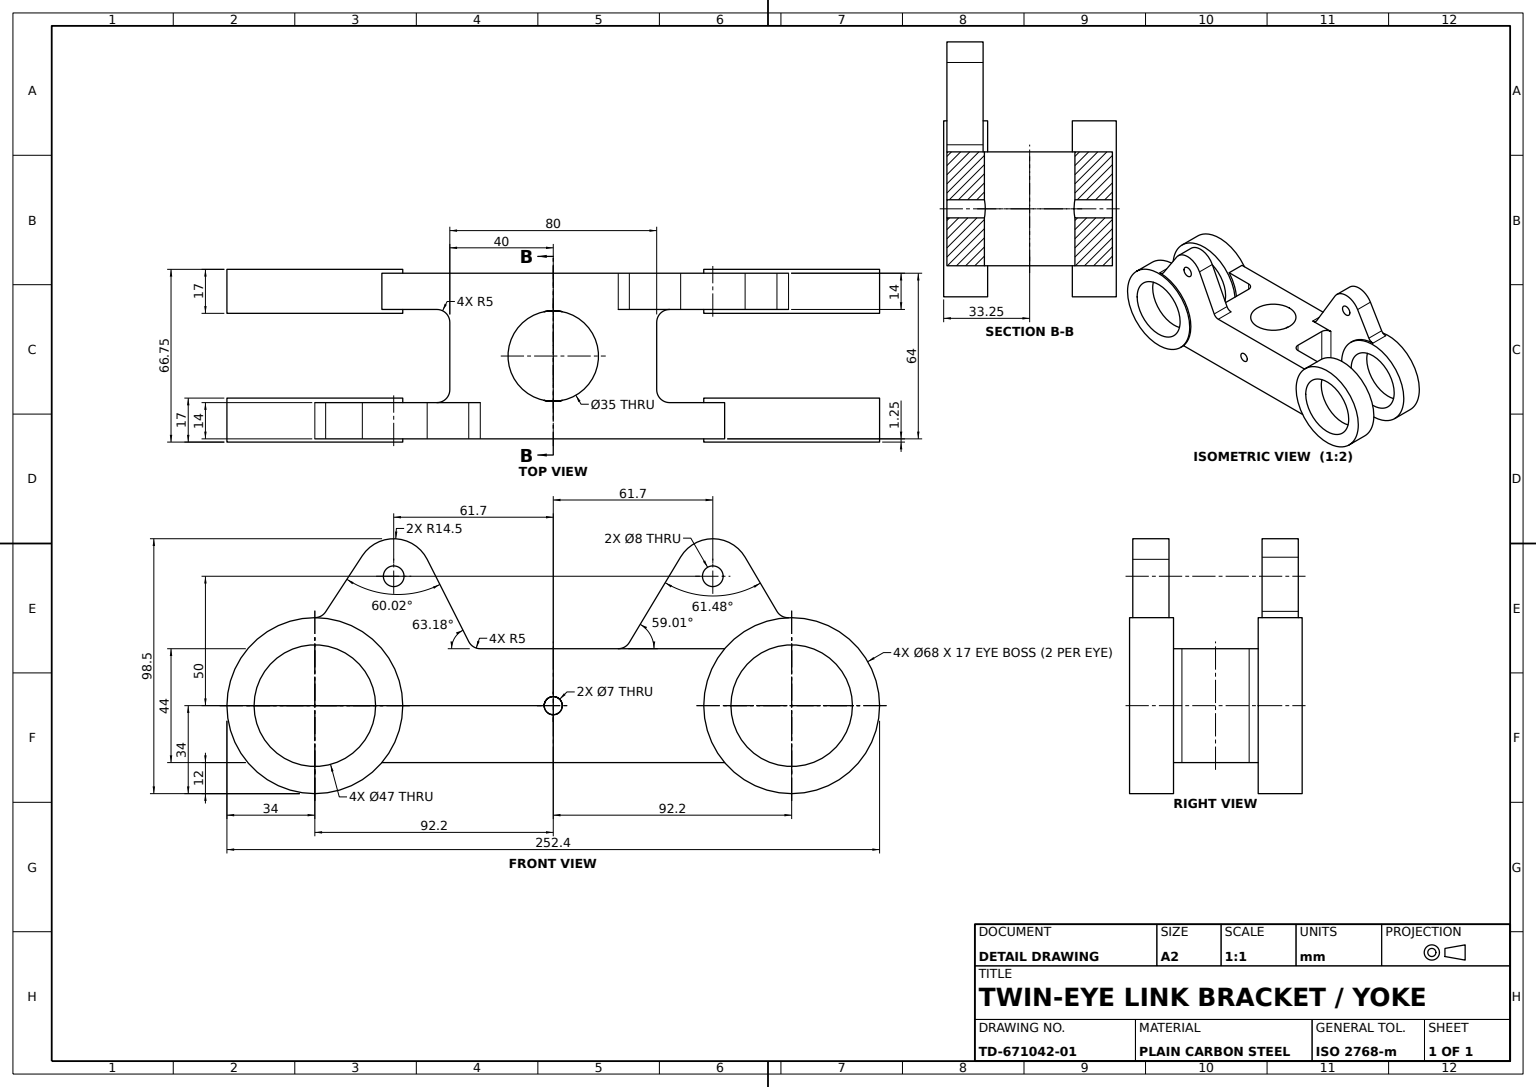
from build123d import *

# Parameters (mm, degrees)
CENTER_BODY_SKETCH_W         = 80
CENTER_BODY_SKETCH_H         = 64
CENTER_BODY_SKETCH_R         = 17.5
CENTER_BODY_DEPTH            = 44
PIVOT_EYES_SKETCH_R          = 34
PIVOT_EYES_SKETCH_R_2        = 23.5
PIVOT_EYES_68X_47_DEPTH      = 15.75
PIVOT_EYES_68X_47_2_DEPTH    = 15.75
EYE_FACE_PADS_SKETCH_R       = 34
EYE_FACE_PADS_SKETCH_R_2     = 23.5
EYE_FACE_PADS_DEPTH          = 1.25
MOUNTING_LUG_A_SKETCH_W      = 27.466221721
MOUNTING_LUG_A_SKETCH_H      = 44
MOUNTING_LUG_A_SKETCH_R      = 4
MOUNTING_LUG_A_DEPTH         = 7
MOUNTING_START               = -14
MOUNTING_LUG_B_SKETCH_R      = 4
MOUNTING_LUG_B_DEPTH         = 14
OFFSET_PIVOT_EYES_SKETCH_R   = 34
OFFSET_PIVOT_EYES_SKETCH_R_2 = 23.5
OFFSET_PIVOT_EYES_DEPTH      = 8.5
CENTER_WEB_SKETCH_W          = 28.251394121
CENTER_WEB_SKETCH_H          = 44
CENTER_WEB_DEPTH             = 14
PIN_HOLE_SKETCH_R            = 3.5
PIN_HOLE_7_DEPTH             = 200
LUG_A_FILLETS_R5_R           = 5
LUG_B_FILLETS_R5_R           = 5


with BuildPart() as part:
    # Center Body Sketch → Center Body (new body)
    with BuildSketch(Plane(origin=(0, 0, 0), x_dir=(1, 0, 0), z_dir=(0, 1, 0))):
        Rectangle(CENTER_BODY_SKETCH_W, CENTER_BODY_SKETCH_H)
        with Locations(Location((0, 0, 0), (0, 0, 270))):
            Circle(CENTER_BODY_SKETCH_R, mode=Mode.SUBTRACT)
    extrude(amount=CENTER_BODY_DEPTH)



with BuildPart() as body_2:
    # Pivot Eyes Sketch → Pivot Eyes Ø68xØ47 (new body)
    with BuildSketch(Plane.XY.offset(32)):
        with Locations((-92.2, 22)):
            Circle(PIVOT_EYES_SKETCH_R)
        with Locations((-92.2, 22)):
            Circle(PIVOT_EYES_SKETCH_R_2, mode=Mode.SUBTRACT)
    extrude(amount=-PIVOT_EYES_68X_47_DEPTH)



with BuildPart() as body_3:
    # Pivot Eyes Sketch → Pivot Eyes _68x_47 2 (new body)
    with BuildSketch(Plane.XY.offset(32)):
        with Locations((92.2, 22)):
            Circle(PIVOT_EYES_SKETCH_R)
        with Locations((92.2, 22)):
            Circle(PIVOT_EYES_SKETCH_R_2, mode=Mode.SUBTRACT)
    extrude(amount=-PIVOT_EYES_68X_47_2_DEPTH)


with BuildPart() as body_2_1:
    add(body_2.part)

    add(body_3.part)  # Eye Face Pads merges body 3
    # Eye Face Pads Sketch → Eye Face Pads (add)
    # profile 1 of 2: a face of its own
    with BuildSketch(Plane.XY.offset(32)):
        with Locations((-92.2, 22)):
            Circle(EYE_FACE_PADS_SKETCH_R)
        with Locations((-92.2, 22)):
            Circle(EYE_FACE_PADS_SKETCH_R_2, mode=Mode.SUBTRACT)
    # profile 2 of 2: a face of its own
    with BuildSketch(Plane.XY.offset(32)):
        with Locations((92.2, 22)):
            Circle(EYE_FACE_PADS_SKETCH_R)
        with Locations((92.2, 22)):
            Circle(EYE_FACE_PADS_SKETCH_R_2, mode=Mode.SUBTRACT)
    extrude(amount=EYE_FACE_PADS_DEPTH)


with BuildPart() as part_1:
    add(part.part)

    add(body_2_1.part)  # Mounting Lug A merges body 2
    # Mounting Lug A Sketch → Mounting Lug A (add, symmetric)
    # profile 1 of 2: a face of its own
    with BuildSketch(Plane.XY.offset(25)):
        with Locations((53.733110861, 22)):
            Rectangle(MOUNTING_LUG_A_SKETCH_W, MOUNTING_LUG_A_SKETCH_H)
    # profile 2 of 2: a face of its own
    with BuildSketch(Plane.XY.offset(25)):
        with BuildLine():
            Line((-40, 44), (-40, 0))
            Line((-40, 0), (-66.277037206, 0))
            ThreePointArc((-66.277037206, 0), (-61.345502759, 36.282856857), (-92.2, 56))
            ThreePointArc((-92.2, 56), (-89.821719025, 56.601843613), (-88.015979336, 58.262488159))
            Line((-88.015979336, 58.262488159), (-73.833659926, 79.93878434))
            ThreePointArc((-73.833659926, 79.93878434), (-60.894229811, 86.47759422), (-48.760320341, 78.543293537))
            Line((-48.760320341, 78.543293537), (-32.680005104, 46.743691884))
            ThreePointArc((-32.680005104, 46.743691884), (-30.837059719, 44.740801685), (-28.218046601, 44))
            Line((-28.218046601, 44), (-40, 44))
        make_face()
        with Locations((-61.7, 72)):
            Circle(MOUNTING_LUG_A_SKETCH_R, mode=Mode.SUBTRACT)
    extrude(amount=MOUNTING_LUG_A_DEPTH, both=True)

    # Mounting Lug B Sketch → Mounting Lug B (add)
    with BuildSketch(Plane(origin=(0, 0, -32), x_dir=(-1, 0, 0), z_dir=(0, 0, -1)).offset(MOUNTING_START)):
        with BuildLine():
            Line((-40, 44), (-25.135268802, 44))
            ThreePointArc((-25.135268802, 44), (-27.59760019, 44.648342369), (-29.421358071, 46.425230346))
            Line((-29.421358071, 46.425230346), (-49.270341118, 79.466831997))
            ThreePointArc((-49.270341118, 79.466831997), (-61.764908832, 86.499854718), (-74.196010179, 79.355251839))
            Line((-74.196010179, 79.355251839), (-86.507393015, 58.439154252))
            ThreePointArc((-86.507393015, 58.439154252), (-88.41197553, 56.591508495), (-90.993751524, 55.978595683))
            ThreePointArc((-90.993751524, 55.978595683), (-61.096956424, 35.733196289), (-66.277037206, 0))
            Line((-66.277037206, 0), (-40, 0))
            Line((-40, 0), (-40, 44))
        make_face()
        with Locations((-61.7, 72)):
            Circle(MOUNTING_LUG_B_SKETCH_R, mode=Mode.SUBTRACT)
    extrude(amount=MOUNTING_LUG_B_DEPTH)

    # Offset Pivot Eyes Sketch → Offset Pivot Eyes (add, symmetric)
    # profile 1 of 2: a face of its own
    with BuildSketch(Plane.XY.offset(-25)):
        with Locations((92.2, 22)):
            Circle(OFFSET_PIVOT_EYES_SKETCH_R)
        with Locations((92.2, 22)):
            Circle(OFFSET_PIVOT_EYES_SKETCH_R_2, mode=Mode.SUBTRACT)
    # profile 2 of 2: a face of its own
    with BuildSketch(Plane.XY.offset(-25)):
        with Locations((-92.2, 22)):
            Circle(OFFSET_PIVOT_EYES_SKETCH_R)
        with Locations((-92.2, 22)):
            Circle(OFFSET_PIVOT_EYES_SKETCH_R_2, mode=Mode.SUBTRACT)
    extrude(amount=OFFSET_PIVOT_EYES_DEPTH, both=True)


with BuildPart() as offset_pivot_eyes_piece_1:
    # of the separate pieces the step leaves, piece 1, a body of its own (offset_pivot_eyes_pieces)
    add(part_1.part.solids().sort_by_distance((126.2, 22, -33.5))[0])



with BuildPart() as offset_pivot_eyes_piece_2:
    # of the separate pieces the step leaves, piece 2, a body of its own (offset_pivot_eyes_pieces)
    add(part_1.part.solids().sort_by_distance((-58.2, 22, -33.5))[0])


with BuildPart() as offset_pivot_eyes_piece_1_1:
    add(offset_pivot_eyes_piece_1.part)

    add(offset_pivot_eyes_piece_2.part)  # Center Web merges Offset Pivot Eyes piece 2
    # Center Web Sketch → Center Web (add)
    with BuildSketch(Plane(origin=(0, 0, -32), x_dir=(-1, 0, 0), z_dir=(0, 0, -1))):
        with Locations((54.125697061, 22)):
            Rectangle(CENTER_WEB_SKETCH_W, CENTER_WEB_SKETCH_H)
    extrude(amount=-CENTER_WEB_DEPTH)

    # Pin Hole Sketch → Pin Hole Ø7 (cut)
    with BuildSketch(Plane(origin=(0, 0, -32), x_dir=(-1, 0, 0), z_dir=(0, 0, -1))):
        with Locations((0, 22)):
            Circle(PIN_HOLE_SKETCH_R)
    extrude(amount=-PIN_HOLE_7_DEPTH, mode=Mode.SUBTRACT)

    # Lug A Fillets R5
    lug_a_fillets_r5_edges = [offset_pivot_eyes_piece_1_1.edges().sort_by_distance(p)[0] for p in [
        (-40, 22, -18),
        (-40, 22, 18),
    ]]
    fillet(lug_a_fillets_r5_edges, radius=LUG_A_FILLETS_R5_R)

    # Lug B Fillets R5
    lug_b_fillets_r5_edges = [offset_pivot_eyes_piece_1_1.edges().sort_by_distance(p)[0] for p in [
        (40, 22, 18),
        (40, 22, -18),
    ]]
    fillet(lug_b_fillets_r5_edges, radius=LUG_B_FILLETS_R5_R)


solid = offset_pivot_eyes_piece_1_1.part
